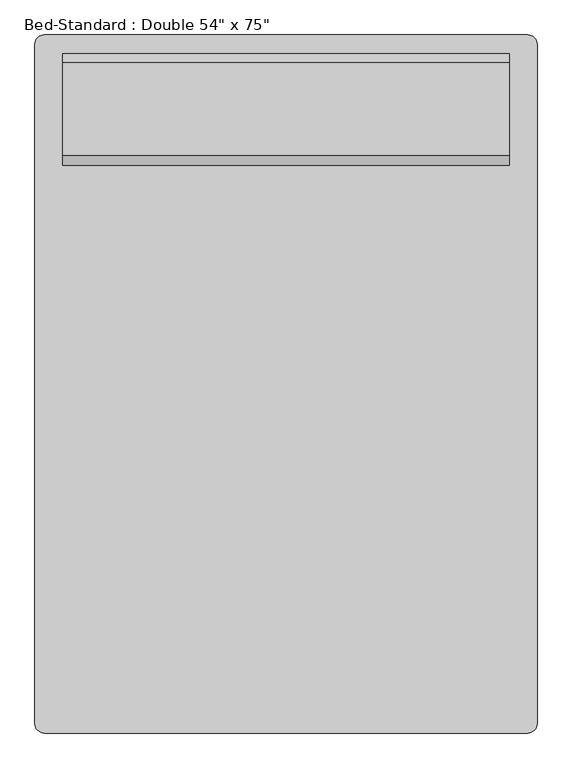
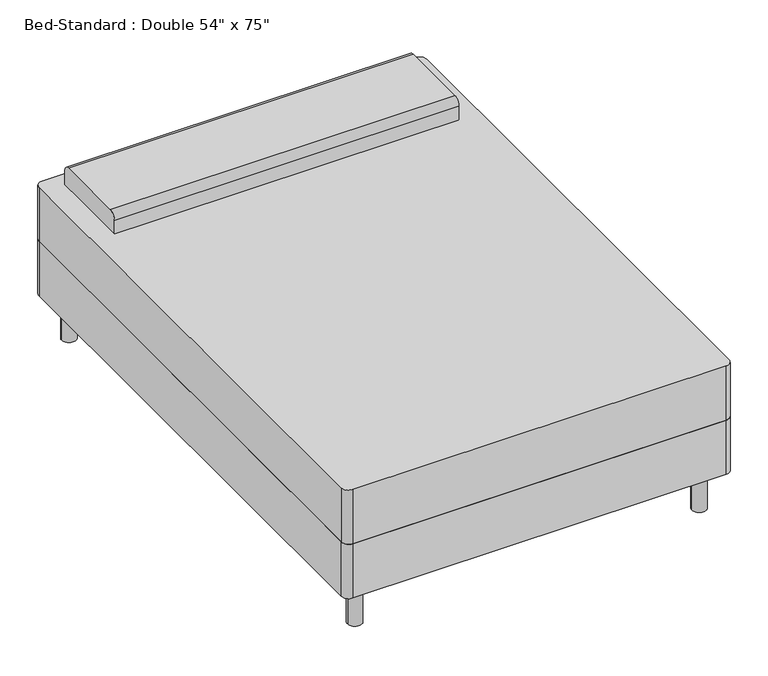
"""IFC4 building model written with IfcOpenShell, lengths in millimetres: furniture geometry."""

from ifc_helpers import new_model, si_unit, point, frame, frame_2d, origin, origin_with_axes, place, context, project, spatial, polyline, circle_curve, trimmed, segment, composite_curve, outline, extrude, source, transform, mapped, element, save


def furniture_0253826f(model_context):
    return source(origin(), model_context, "Body", "SweptSolid", [
        extrude(outline(composite_curve([segment(polyline([(-414.3114754, -972.695082), (-414.3114754, 881.504918)]), True, "CONTINUOUS"), segment(trimmed(circle_curve(frame_2d((-388.9114754, 881.504918)), 25.4), [point((-414.3114754, 881.504918))], [point((-388.9114754, 906.904918))], False, "CARTESIAN"), True, "CONTINUOUS"), segment(polyline([(-388.9114754, 906.904918), (931.8885246, 906.904918)]), True, "CONTINUOUS"), segment(trimmed(circle_curve(frame_2d((931.8885246, 881.504918)), 25.4), [point((931.8885246, 906.904918))], [point((957.2885246, 881.504918))], False, "CARTESIAN"), True, "CONTINUOUS"), segment(polyline([(957.2885246, 881.504918), (957.2885246, -972.695082)]), True, "CONTINUOUS"), segment(trimmed(circle_curve(frame_2d((931.8885246, -972.695082)), 25.4), [point((957.2885246, -972.695082))], [point((931.8885246, -998.095082))], False, "CARTESIAN"), True, "CONTINUOUS"), segment(polyline([(931.8885246, -998.095082), (-388.9114754, -998.095082)]), True, "CONTINUOUS"), segment(trimmed(circle_curve(frame_2d((-388.9114754, -972.695082)), 25.4), [point((-388.9114754, -998.095082))], [point((-414.3114754, -972.695082))], False, "CARTESIAN"), True, "CONTINUOUS")], self_intersect=False)), frame((0.0, 0.0, 152.4), z_axis=(0.0, 0.0, 1.0), x_axis=(1.0, 0.0, 0.0)), (0.0, 0.0, 1.0), 203.2),
        extrude(outline(composite_curve([segment(polyline([(551.304918, 558.8), (551.304918, 609.6)]), True, "CONTINUOUS"), segment(trimmed(circle_curve(frame_2d((576.704918, 609.6)), 25.4), [point((551.304918, 609.6))], [point((576.704918, 635.0))], False, "CARTESIAN"), True, "CONTINUOUS"), segment(polyline([(576.704918, 635.0), (830.704918, 635.0)]), True, "CONTINUOUS"), segment(trimmed(circle_curve(frame_2d((830.704918, 609.6)), 25.4), [point((830.704918, 635.0))], [point((856.104918, 609.6))], False, "CARTESIAN"), True, "CONTINUOUS"), segment(polyline([(856.104918, 609.6), (856.104918, 558.8), (551.304918, 558.8)]), True, "CONTINUOUS")], self_intersect=False)), frame((-338.1114754, 0.0, 0.0), z_axis=(1.0, 0.0, 0.0), x_axis=(0.0, 1.0, 0.0)), (0.0, 0.0, 1.0), 1219.2),
        extrude(outline(composite_curve([segment(trimmed(circle_curve(frame_2d((-338.1114754, 830.704918)), 25.4), [point((-363.5114754, 830.704918))], [point((-312.7114754, 830.704918))], False, "CARTESIAN"), True, "CONTINUOUS"), segment(trimmed(circle_curve(frame_2d((-338.1114754, 830.704918)), 25.4), [point((-312.7114754, 830.704918))], [point((-363.5114754, 830.704918))], False, "CARTESIAN"), True, "CONTINUOUS")], self_intersect=False)), origin_with_axes(), (0.0, 0.0, 1.0), 152.4),
        extrude(outline(composite_curve([segment(trimmed(circle_curve(frame_2d((881.0885246, 830.704918)), 25.4), [point((855.6885246, 830.704918))], [point((906.4885246, 830.704918))], False, "CARTESIAN"), True, "CONTINUOUS"), segment(trimmed(circle_curve(frame_2d((881.0885246, 830.704918)), 25.4), [point((906.4885246, 830.704918))], [point((855.6885246, 830.704918))], False, "CARTESIAN"), True, "CONTINUOUS")], self_intersect=False)), origin_with_axes(), (0.0, 0.0, 1.0), 152.4),
        extrude(outline(composite_curve([segment(trimmed(circle_curve(frame_2d((881.0885246, -921.895082)), 25.4), [point((855.6885246, -921.895082))], [point((906.4885246, -921.895082))], False, "CARTESIAN"), True, "CONTINUOUS"), segment(trimmed(circle_curve(frame_2d((881.0885246, -921.895082)), 25.4), [point((906.4885246, -921.895082))], [point((855.6885246, -921.895082))], False, "CARTESIAN"), True, "CONTINUOUS")], self_intersect=False)), origin_with_axes(), (0.0, 0.0, 1.0), 152.4),
        extrude(outline(composite_curve([segment(trimmed(circle_curve(frame_2d((-338.1114754, -921.895082)), 25.4), [point((-363.5114754, -921.895082))], [point((-312.7114754, -921.895082))], False, "CARTESIAN"), True, "CONTINUOUS"), segment(trimmed(circle_curve(frame_2d((-338.1114754, -921.895082)), 25.4), [point((-312.7114754, -921.895082))], [point((-363.5114754, -921.895082))], False, "CARTESIAN"), True, "CONTINUOUS")], self_intersect=False)), origin_with_axes(), (0.0, 0.0, 1.0), 152.4),
        extrude(outline(composite_curve([segment(polyline([(-388.9114754, 906.904918), (931.8885246, 906.904918)]), True, "CONTINUOUS"), segment(trimmed(circle_curve(frame_2d((931.8885246, 881.504918)), 25.4), [point((931.8885246, 906.904918))], [point((957.2885246, 881.504918))], False, "CARTESIAN"), True, "CONTINUOUS"), segment(polyline([(957.2885246, 881.504918), (957.2885246, -972.695082)]), True, "CONTINUOUS"), segment(trimmed(circle_curve(frame_2d((931.8885246, -972.695082)), 25.4), [point((957.2885246, -972.695082))], [point((931.8885246, -998.095082))], False, "CARTESIAN"), True, "CONTINUOUS"), segment(polyline([(931.8885246, -998.095082), (-388.9114754, -998.095082)]), True, "CONTINUOUS"), segment(trimmed(circle_curve(frame_2d((-388.9114754, -972.695082)), 25.4), [point((-388.9114754, -998.095082))], [point((-414.3114754, -972.695082))], False, "CARTESIAN"), True, "CONTINUOUS"), segment(polyline([(-414.3114754, -972.695082), (-414.3114754, 881.504918)]), True, "CONTINUOUS"), segment(trimmed(circle_curve(frame_2d((-388.9114754, 881.504918)), 25.4), [point((-414.3114754, 881.504918))], [point((-388.9114754, 906.904918))], False, "CARTESIAN"), True, "CONTINUOUS")], self_intersect=False)), frame((0.0, 0.0, 355.6), z_axis=(0.0, 0.0, 1.0), x_axis=(1.0, 0.0, 0.0)), (0.0, 0.0, 1.0), 203.2),
    ])


if __name__ == "__main__":
    model = new_model("IFC4")
    model_context = context("Model", 3, world=origin())
    ifc_project = project(units=[si_unit("LENGTHUNIT", "METRE", prefix="MILLI")], contexts=[model_context])
    site = spatial("IfcSite", under=ifc_project)
    building = spatial("IfcBuilding", under=site)
    placement = place(None, origin())
    furniture_shape = furniture_0253826f(model_context)
    element("IfcFurniture", 1, ObjectType="Bed-Standard : Double 54\" x 75\"", at=placement, inside=building, context=model_context, shape_type="MappedRepresentation", body=[
        mapped(furniture_shape, transform((0.0, 0.0, 0.0), x_axis=(1.0, 0.0, 0.0), y_axis=(0.0, 1.0, 0.0), z_axis=(0.0, 0.0, 1.0))),
    ])
    save(model, "model.ifc")

# Revit data of these elements
# Type "Bed-Standard : Double 54\" x 75\""
#   Assembly Code = "E2020200"
#   Length = 6' - 3"
#   Width = 4' - 6"
#   Leg Material = Steel, Chrome Plated
#   Mattress Material = Textile - Bamboo Weave
#   Default Elevation = 0
# Element 1 (IfcFurniture, "Bed-Standard : Double 54\" x 75\"")
#   Materials on its faces: "Linen, White", "Steel, Chrome Plated"
# Materials
#   "Steel, Chrome Plated": class "Metal", colour RGB 17 17 17, transparency 0, Description = "Chromiuim plated steel", Cost = 0
#   "Textile - Bamboo Weave": class "Fabric", colour RGB 246 223 112, transparency 0
#   "Linen, White": class "Textile", colour RGB 247 247 239, transparency 0, Description = "Linen, white", Cost = 0
